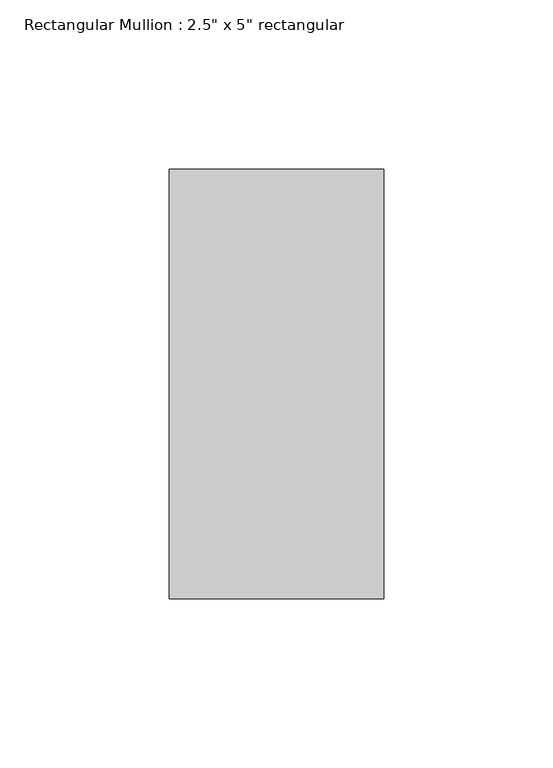
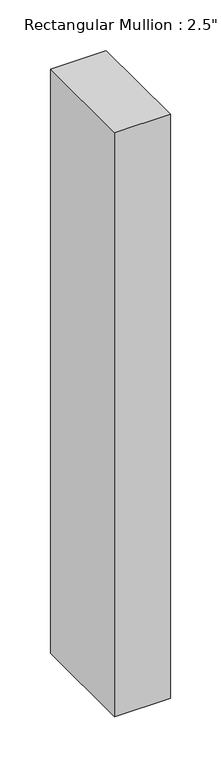
"""IFC4 building model written with IfcOpenShell, lengths in millimetres: member geometry."""

from ifc_helpers import new_model, si_unit, frame, origin, place, context, project, spatial, polyline, outline, extrude, source, transform, mapped, element, save


def member_0d9ba275(model_context):
    return source(origin(), model_context, "Body", "SweptSolid", [
        extrude(outline(polyline([(0.0, 63.5), (0.0, -63.5), (-63.5, -63.5), (-63.5, 63.5), (0.0, 63.5)])), frame((0.0, 0.0, -704.8281229), z_axis=(0.0, 0.0, 1.0), x_axis=(1.0, 0.0, 0.0)), (0.0, 0.0, 1.0), 704.8281229),
    ])


if __name__ == "__main__":
    model = new_model("IFC4")
    model_context = context("Model", 3, world=origin())
    ifc_project = project(units=[si_unit("LENGTHUNIT", "METRE", prefix="MILLI")], contexts=[model_context])
    site = spatial("IfcSite", under=ifc_project)
    building = spatial("IfcBuilding", under=site)
    placement = place(None, origin())
    member_shape = member_0d9ba275(model_context)
    element("IfcMember", 1, ObjectType="Rectangular Mullion : 2.5\" x 5\" rectangular", at=placement, inside=building, context=model_context, shape_type="MappedRepresentation", body=[
        mapped(member_shape, transform((0.0, 0.0, 0.0), x_axis=(1.0, 0.0, 0.0), y_axis=(0.0, 1.0, 0.0), z_axis=(0.0, 0.0, 1.0))),
    ])
    save(model, "model.ifc")

# Revit data of these elements
# Type "Rectangular Mullion : 2.5\" x 5\" rectangular"
#   built-in parameter 1007304 = 0.416667 (stored number, unit not read)
#   built-in parameter 1007301 = 0.104167 (stored number, unit not read)
#   built-in parameter 1007300 = 0.104167 (stored number, unit not read)
# Element 1 (IfcMember, "Rectangular Mullion : 2.5\" x 5\" rectangular")
#   Materials on its faces: "Aluminum"
# Materials
#   "Aluminum": class "Metal", colour RGB 247 247 247, transparency 0, Description = "Aluminum 6061", Cost = 0
